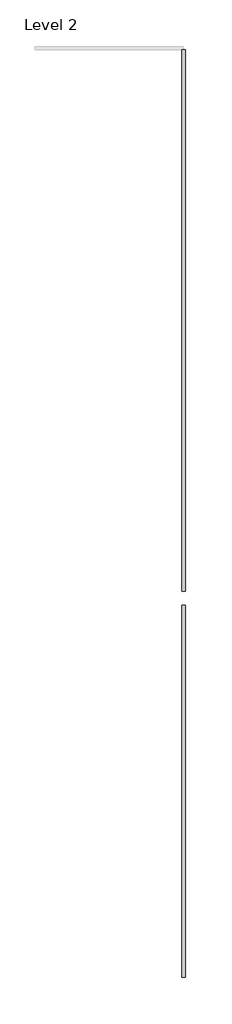
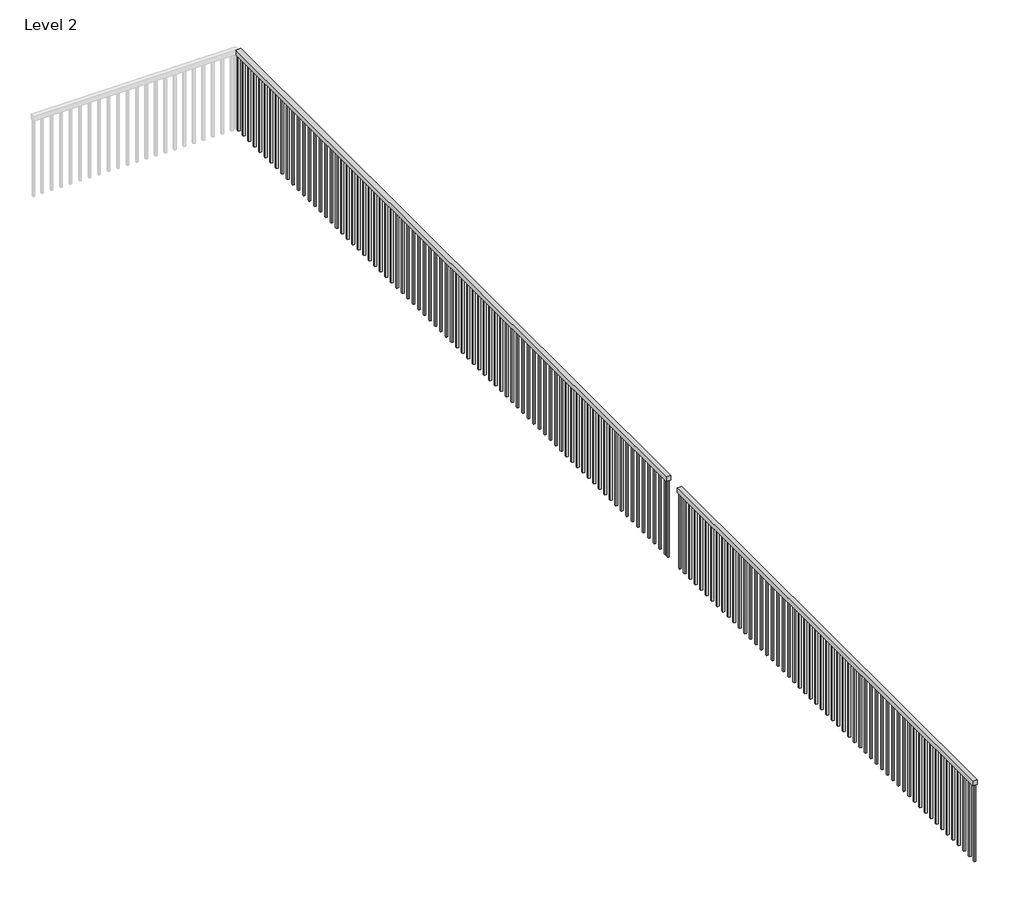
# One storey, part 4 of 5: 2 railings.
"""IFC4 building model written with IfcOpenShell, lengths in millimetres."""

from ifc_helpers import new_model, si_unit, frame, origin, place, context, project, spatial, polyline, outline, extrude, element, save

model = new_model("IFC4")

# Units and contexts
model_context = context("Model", 3, world=origin())
ifc_project = project(units=[si_unit("LENGTHUNIT", "METRE", prefix="MILLI")], contexts=[model_context])

# Site, building, storey
site = spatial("IfcSite", under=ifc_project)
building = spatial("IfcBuilding", under=site)
storey = spatial("IfcBuildingStorey", under=building, Name="Level 2", Elevation=3048.0)

# Railings
placement = place(None, origin())
element("IfcRailing", 1, ObjectType="Handrail - Rectangular", at=placement, inside=storey, context=model_context, shape_type="SweptSolid", body=[
    extrude(outline(polyline([(16296.0289933, 16349.0250499), (16346.8289933, 16349.0250499), (16346.8289933, 8367.8237525), (16296.0289933, 8367.8237525), (16296.0289933, 16349.0250499)])), frame((0.0, 0.0, 3911.6), z_axis=(0.0, 0.0, 1.0), x_axis=(1.0, 0.0, 0.0)), (0.0, 0.0, 1.0), 50.8),
    extrude(outline(polyline([(16311.9039933, 8433.7500499), (16330.9539933, 8433.7500499), (16330.9539933, 8414.7000499), (16311.9039933, 8414.7000499), (16311.9039933, 8433.7500499)])), frame((0.0, 0.0, 3048.0), z_axis=(0.0, 0.0, 1.0), x_axis=(1.0, 0.0, 0.0)), (0.0, 0.0, 1.0), 863.6),
    extrude(outline(polyline([(16311.9039933, 8535.3500499), (16330.9539933, 8535.3500499), (16330.9539933, 8516.3000499), (16311.9039933, 8516.3000499), (16311.9039933, 8535.3500499)])), frame((0.0, 0.0, 3048.0), z_axis=(0.0, 0.0, 1.0), x_axis=(1.0, 0.0, 0.0)), (0.0, 0.0, 1.0), 863.6),
    extrude(outline(polyline([(16311.9039933, 8636.9500499), (16330.9539933, 8636.9500499), (16330.9539933, 8617.9000499), (16311.9039933, 8617.9000499), (16311.9039933, 8636.9500499)])), frame((0.0, 0.0, 3048.0), z_axis=(0.0, 0.0, 1.0), x_axis=(1.0, 0.0, 0.0)), (0.0, 0.0, 1.0), 863.6),
    extrude(outline(polyline([(16311.9039933, 8738.5500499), (16330.9539933, 8738.5500499), (16330.9539933, 8719.5000499), (16311.9039933, 8719.5000499), (16311.9039933, 8738.5500499)])), frame((0.0, 0.0, 3048.0), z_axis=(0.0, 0.0, 1.0), x_axis=(1.0, 0.0, 0.0)), (0.0, 0.0, 1.0), 863.6),
    extrude(outline(polyline([(16311.9039933, 8840.1500499), (16330.9539933, 8840.1500499), (16330.9539933, 8821.1000499), (16311.9039933, 8821.1000499), (16311.9039933, 8840.1500499)])), frame((0.0, 0.0, 3048.0), z_axis=(0.0, 0.0, 1.0), x_axis=(1.0, 0.0, 0.0)), (0.0, 0.0, 1.0), 863.6),
    extrude(outline(polyline([(16311.9039933, 8941.7500499), (16330.9539933, 8941.7500499), (16330.9539933, 8922.7000499), (16311.9039933, 8922.7000499), (16311.9039933, 8941.7500499)])), frame((0.0, 0.0, 3048.0), z_axis=(0.0, 0.0, 1.0), x_axis=(1.0, 0.0, 0.0)), (0.0, 0.0, 1.0), 863.6),
    extrude(outline(polyline([(16311.9039933, 9043.3500499), (16330.9539933, 9043.3500499), (16330.9539933, 9024.3000499), (16311.9039933, 9024.3000499), (16311.9039933, 9043.3500499)])), frame((0.0, 0.0, 3048.0), z_axis=(0.0, 0.0, 1.0), x_axis=(1.0, 0.0, 0.0)), (0.0, 0.0, 1.0), 863.6),
    extrude(outline(polyline([(16311.9039933, 9144.9500499), (16330.9539933, 9144.9500499), (16330.9539933, 9125.9000499), (16311.9039933, 9125.9000499), (16311.9039933, 9144.9500499)])), frame((0.0, 0.0, 3048.0), z_axis=(0.0, 0.0, 1.0), x_axis=(1.0, 0.0, 0.0)), (0.0, 0.0, 1.0), 863.6),
    extrude(outline(polyline([(16311.9039933, 9246.5500499), (16330.9539933, 9246.5500499), (16330.9539933, 9227.5000499), (16311.9039933, 9227.5000499), (16311.9039933, 9246.5500499)])), frame((0.0, 0.0, 3048.0), z_axis=(0.0, 0.0, 1.0), x_axis=(1.0, 0.0, 0.0)), (0.0, 0.0, 1.0), 863.6),
    extrude(outline(polyline([(16311.9039933, 9348.1500499), (16330.9539933, 9348.1500499), (16330.9539933, 9329.1000499), (16311.9039933, 9329.1000499), (16311.9039933, 9348.1500499)])), frame((0.0, 0.0, 3048.0), z_axis=(0.0, 0.0, 1.0), x_axis=(1.0, 0.0, 0.0)), (0.0, 0.0, 1.0), 863.6),
    extrude(outline(polyline([(16311.9039933, 9449.7500499), (16330.9539933, 9449.7500499), (16330.9539933, 9430.7000499), (16311.9039933, 9430.7000499), (16311.9039933, 9449.7500499)])), frame((0.0, 0.0, 3048.0), z_axis=(0.0, 0.0, 1.0), x_axis=(1.0, 0.0, 0.0)), (0.0, 0.0, 1.0), 863.6),
    extrude(outline(polyline([(16311.9039933, 9551.3500499), (16330.9539933, 9551.3500499), (16330.9539933, 9532.3000499), (16311.9039933, 9532.3000499), (16311.9039933, 9551.3500499)])), frame((0.0, 0.0, 3048.0), z_axis=(0.0, 0.0, 1.0), x_axis=(1.0, 0.0, 0.0)), (0.0, 0.0, 1.0), 863.6),
    extrude(outline(polyline([(16311.9039933, 9652.9500499), (16330.9539933, 9652.9500499), (16330.9539933, 9633.9000499), (16311.9039933, 9633.9000499), (16311.9039933, 9652.9500499)])), frame((0.0, 0.0, 3048.0), z_axis=(0.0, 0.0, 1.0), x_axis=(1.0, 0.0, 0.0)), (0.0, 0.0, 1.0), 863.6),
    extrude(outline(polyline([(16311.9039933, 9754.5500499), (16330.9539933, 9754.5500499), (16330.9539933, 9735.5000499), (16311.9039933, 9735.5000499), (16311.9039933, 9754.5500499)])), frame((0.0, 0.0, 3048.0), z_axis=(0.0, 0.0, 1.0), x_axis=(1.0, 0.0, 0.0)), (0.0, 0.0, 1.0), 863.6),
    extrude(outline(polyline([(16311.9039933, 9856.1500499), (16330.9539933, 9856.1500499), (16330.9539933, 9837.1000499), (16311.9039933, 9837.1000499), (16311.9039933, 9856.1500499)])), frame((0.0, 0.0, 3048.0), z_axis=(0.0, 0.0, 1.0), x_axis=(1.0, 0.0, 0.0)), (0.0, 0.0, 1.0), 863.6),
    extrude(outline(polyline([(16311.9039933, 9957.7500499), (16330.9539933, 9957.7500499), (16330.9539933, 9938.7000499), (16311.9039933, 9938.7000499), (16311.9039933, 9957.7500499)])), frame((0.0, 0.0, 3048.0), z_axis=(0.0, 0.0, 1.0), x_axis=(1.0, 0.0, 0.0)), (0.0, 0.0, 1.0), 863.6),
    extrude(outline(polyline([(16311.9039933, 10059.3500499), (16330.9539933, 10059.3500499), (16330.9539933, 10040.3000499), (16311.9039933, 10040.3000499), (16311.9039933, 10059.3500499)])), frame((0.0, 0.0, 3048.0), z_axis=(0.0, 0.0, 1.0), x_axis=(1.0, 0.0, 0.0)), (0.0, 0.0, 1.0), 863.6),
    extrude(outline(polyline([(16311.9039933, 10160.9500499), (16330.9539933, 10160.9500499), (16330.9539933, 10141.9000499), (16311.9039933, 10141.9000499), (16311.9039933, 10160.9500499)])), frame((0.0, 0.0, 3048.0), z_axis=(0.0, 0.0, 1.0), x_axis=(1.0, 0.0, 0.0)), (0.0, 0.0, 1.0), 863.6),
    extrude(outline(polyline([(16311.9039933, 10262.5500499), (16330.9539933, 10262.5500499), (16330.9539933, 10243.5000499), (16311.9039933, 10243.5000499), (16311.9039933, 10262.5500499)])), frame((0.0, 0.0, 3048.0), z_axis=(0.0, 0.0, 1.0), x_axis=(1.0, 0.0, 0.0)), (0.0, 0.0, 1.0), 863.6),
    extrude(outline(polyline([(16311.9039933, 10364.1500499), (16330.9539933, 10364.1500499), (16330.9539933, 10345.1000499), (16311.9039933, 10345.1000499), (16311.9039933, 10364.1500499)])), frame((0.0, 0.0, 3048.0), z_axis=(0.0, 0.0, 1.0), x_axis=(1.0, 0.0, 0.0)), (0.0, 0.0, 1.0), 863.6),
    extrude(outline(polyline([(16311.9039933, 10465.7500499), (16330.9539933, 10465.7500499), (16330.9539933, 10446.7000499), (16311.9039933, 10446.7000499), (16311.9039933, 10465.7500499)])), frame((0.0, 0.0, 3048.0), z_axis=(0.0, 0.0, 1.0), x_axis=(1.0, 0.0, 0.0)), (0.0, 0.0, 1.0), 863.6),
    extrude(outline(polyline([(16311.9039933, 10567.3500499), (16330.9539933, 10567.3500499), (16330.9539933, 10548.3000499), (16311.9039933, 10548.3000499), (16311.9039933, 10567.3500499)])), frame((0.0, 0.0, 3048.0), z_axis=(0.0, 0.0, 1.0), x_axis=(1.0, 0.0, 0.0)), (0.0, 0.0, 1.0), 863.6),
    extrude(outline(polyline([(16311.9039933, 10668.9500499), (16330.9539933, 10668.9500499), (16330.9539933, 10649.9000499), (16311.9039933, 10649.9000499), (16311.9039933, 10668.9500499)])), frame((0.0, 0.0, 3048.0), z_axis=(0.0, 0.0, 1.0), x_axis=(1.0, 0.0, 0.0)), (0.0, 0.0, 1.0), 863.6),
    extrude(outline(polyline([(16311.9039933, 10770.5500499), (16330.9539933, 10770.5500499), (16330.9539933, 10751.5000499), (16311.9039933, 10751.5000499), (16311.9039933, 10770.5500499)])), frame((0.0, 0.0, 3048.0), z_axis=(0.0, 0.0, 1.0), x_axis=(1.0, 0.0, 0.0)), (0.0, 0.0, 1.0), 863.6),
    extrude(outline(polyline([(16311.9039933, 10872.1500499), (16330.9539933, 10872.1500499), (16330.9539933, 10853.1000499), (16311.9039933, 10853.1000499), (16311.9039933, 10872.1500499)])), frame((0.0, 0.0, 3048.0), z_axis=(0.0, 0.0, 1.0), x_axis=(1.0, 0.0, 0.0)), (0.0, 0.0, 1.0), 863.6),
    extrude(outline(polyline([(16311.9039933, 10973.7500499), (16330.9539933, 10973.7500499), (16330.9539933, 10954.7000499), (16311.9039933, 10954.7000499), (16311.9039933, 10973.7500499)])), frame((0.0, 0.0, 3048.0), z_axis=(0.0, 0.0, 1.0), x_axis=(1.0, 0.0, 0.0)), (0.0, 0.0, 1.0), 863.6),
    extrude(outline(polyline([(16311.9039933, 11075.3500499), (16330.9539933, 11075.3500499), (16330.9539933, 11056.3000499), (16311.9039933, 11056.3000499), (16311.9039933, 11075.3500499)])), frame((0.0, 0.0, 3048.0), z_axis=(0.0, 0.0, 1.0), x_axis=(1.0, 0.0, 0.0)), (0.0, 0.0, 1.0), 863.6),
    extrude(outline(polyline([(16311.9039933, 11176.9500499), (16330.9539933, 11176.9500499), (16330.9539933, 11157.9000499), (16311.9039933, 11157.9000499), (16311.9039933, 11176.9500499)])), frame((0.0, 0.0, 3048.0), z_axis=(0.0, 0.0, 1.0), x_axis=(1.0, 0.0, 0.0)), (0.0, 0.0, 1.0), 863.6),
    extrude(outline(polyline([(16311.9039933, 11278.5500499), (16330.9539933, 11278.5500499), (16330.9539933, 11259.5000499), (16311.9039933, 11259.5000499), (16311.9039933, 11278.5500499)])), frame((0.0, 0.0, 3048.0), z_axis=(0.0, 0.0, 1.0), x_axis=(1.0, 0.0, 0.0)), (0.0, 0.0, 1.0), 863.6),
    extrude(outline(polyline([(16311.9039933, 11380.1500499), (16330.9539933, 11380.1500499), (16330.9539933, 11361.1000499), (16311.9039933, 11361.1000499), (16311.9039933, 11380.1500499)])), frame((0.0, 0.0, 3048.0), z_axis=(0.0, 0.0, 1.0), x_axis=(1.0, 0.0, 0.0)), (0.0, 0.0, 1.0), 863.6),
    extrude(outline(polyline([(16311.9039933, 11481.7500499), (16330.9539933, 11481.7500499), (16330.9539933, 11462.7000499), (16311.9039933, 11462.7000499), (16311.9039933, 11481.7500499)])), frame((0.0, 0.0, 3048.0), z_axis=(0.0, 0.0, 1.0), x_axis=(1.0, 0.0, 0.0)), (0.0, 0.0, 1.0), 863.6),
    extrude(outline(polyline([(16311.9039933, 11583.3500499), (16330.9539933, 11583.3500499), (16330.9539933, 11564.3000499), (16311.9039933, 11564.3000499), (16311.9039933, 11583.3500499)])), frame((0.0, 0.0, 3048.0), z_axis=(0.0, 0.0, 1.0), x_axis=(1.0, 0.0, 0.0)), (0.0, 0.0, 1.0), 863.6),
    extrude(outline(polyline([(16311.9039933, 11684.9500499), (16330.9539933, 11684.9500499), (16330.9539933, 11665.9000499), (16311.9039933, 11665.9000499), (16311.9039933, 11684.9500499)])), frame((0.0, 0.0, 3048.0), z_axis=(0.0, 0.0, 1.0), x_axis=(1.0, 0.0, 0.0)), (0.0, 0.0, 1.0), 863.6),
    extrude(outline(polyline([(16311.9039933, 11786.5500499), (16330.9539933, 11786.5500499), (16330.9539933, 11767.5000499), (16311.9039933, 11767.5000499), (16311.9039933, 11786.5500499)])), frame((0.0, 0.0, 3048.0), z_axis=(0.0, 0.0, 1.0), x_axis=(1.0, 0.0, 0.0)), (0.0, 0.0, 1.0), 863.6),
    extrude(outline(polyline([(16311.9039933, 11888.1500499), (16330.9539933, 11888.1500499), (16330.9539933, 11869.1000499), (16311.9039933, 11869.1000499), (16311.9039933, 11888.1500499)])), frame((0.0, 0.0, 3048.0), z_axis=(0.0, 0.0, 1.0), x_axis=(1.0, 0.0, 0.0)), (0.0, 0.0, 1.0), 863.6),
    extrude(outline(polyline([(16311.9039933, 11989.7500499), (16330.9539933, 11989.7500499), (16330.9539933, 11970.7000499), (16311.9039933, 11970.7000499), (16311.9039933, 11989.7500499)])), frame((0.0, 0.0, 3048.0), z_axis=(0.0, 0.0, 1.0), x_axis=(1.0, 0.0, 0.0)), (0.0, 0.0, 1.0), 863.6),
    extrude(outline(polyline([(16311.9039933, 12091.3500499), (16330.9539933, 12091.3500499), (16330.9539933, 12072.3000499), (16311.9039933, 12072.3000499), (16311.9039933, 12091.3500499)])), frame((0.0, 0.0, 3048.0), z_axis=(0.0, 0.0, 1.0), x_axis=(1.0, 0.0, 0.0)), (0.0, 0.0, 1.0), 863.6),
    extrude(outline(polyline([(16311.9039933, 12192.9500499), (16330.9539933, 12192.9500499), (16330.9539933, 12173.9000499), (16311.9039933, 12173.9000499), (16311.9039933, 12192.9500499)])), frame((0.0, 0.0, 3048.0), z_axis=(0.0, 0.0, 1.0), x_axis=(1.0, 0.0, 0.0)), (0.0, 0.0, 1.0), 863.6),
    extrude(outline(polyline([(16311.9039933, 12294.5500499), (16330.9539933, 12294.5500499), (16330.9539933, 12275.5000499), (16311.9039933, 12275.5000499), (16311.9039933, 12294.5500499)])), frame((0.0, 0.0, 3048.0), z_axis=(0.0, 0.0, 1.0), x_axis=(1.0, 0.0, 0.0)), (0.0, 0.0, 1.0), 863.6),
    extrude(outline(polyline([(16311.9039933, 12396.1500499), (16330.9539933, 12396.1500499), (16330.9539933, 12377.1000499), (16311.9039933, 12377.1000499), (16311.9039933, 12396.1500499)])), frame((0.0, 0.0, 3048.0), z_axis=(0.0, 0.0, 1.0), x_axis=(1.0, 0.0, 0.0)), (0.0, 0.0, 1.0), 863.6),
    extrude(outline(polyline([(16311.9039933, 12497.7500499), (16330.9539933, 12497.7500499), (16330.9539933, 12478.7000499), (16311.9039933, 12478.7000499), (16311.9039933, 12497.7500499)])), frame((0.0, 0.0, 3048.0), z_axis=(0.0, 0.0, 1.0), x_axis=(1.0, 0.0, 0.0)), (0.0, 0.0, 1.0), 863.6),
    extrude(outline(polyline([(16311.9039933, 12599.3500499), (16330.9539933, 12599.3500499), (16330.9539933, 12580.3000499), (16311.9039933, 12580.3000499), (16311.9039933, 12599.3500499)])), frame((0.0, 0.0, 3048.0), z_axis=(0.0, 0.0, 1.0), x_axis=(1.0, 0.0, 0.0)), (0.0, 0.0, 1.0), 863.6),
    extrude(outline(polyline([(16311.9039933, 12700.9500499), (16330.9539933, 12700.9500499), (16330.9539933, 12681.9000499), (16311.9039933, 12681.9000499), (16311.9039933, 12700.9500499)])), frame((0.0, 0.0, 3048.0), z_axis=(0.0, 0.0, 1.0), x_axis=(1.0, 0.0, 0.0)), (0.0, 0.0, 1.0), 863.6),
    extrude(outline(polyline([(16311.9039933, 12802.5500499), (16330.9539933, 12802.5500499), (16330.9539933, 12783.5000499), (16311.9039933, 12783.5000499), (16311.9039933, 12802.5500499)])), frame((0.0, 0.0, 3048.0), z_axis=(0.0, 0.0, 1.0), x_axis=(1.0, 0.0, 0.0)), (0.0, 0.0, 1.0), 863.6),
    extrude(outline(polyline([(16311.9039933, 12904.1500499), (16330.9539933, 12904.1500499), (16330.9539933, 12885.1000499), (16311.9039933, 12885.1000499), (16311.9039933, 12904.1500499)])), frame((0.0, 0.0, 3048.0), z_axis=(0.0, 0.0, 1.0), x_axis=(1.0, 0.0, 0.0)), (0.0, 0.0, 1.0), 863.6),
    extrude(outline(polyline([(16311.9039933, 13005.7500499), (16330.9539933, 13005.7500499), (16330.9539933, 12986.7000499), (16311.9039933, 12986.7000499), (16311.9039933, 13005.7500499)])), frame((0.0, 0.0, 3048.0), z_axis=(0.0, 0.0, 1.0), x_axis=(1.0, 0.0, 0.0)), (0.0, 0.0, 1.0), 863.6),
    extrude(outline(polyline([(16311.9039933, 13107.3500499), (16330.9539933, 13107.3500499), (16330.9539933, 13088.3000499), (16311.9039933, 13088.3000499), (16311.9039933, 13107.3500499)])), frame((0.0, 0.0, 3048.0), z_axis=(0.0, 0.0, 1.0), x_axis=(1.0, 0.0, 0.0)), (0.0, 0.0, 1.0), 863.6),
    extrude(outline(polyline([(16311.9039933, 13208.9500499), (16330.9539933, 13208.9500499), (16330.9539933, 13189.9000499), (16311.9039933, 13189.9000499), (16311.9039933, 13208.9500499)])), frame((0.0, 0.0, 3048.0), z_axis=(0.0, 0.0, 1.0), x_axis=(1.0, 0.0, 0.0)), (0.0, 0.0, 1.0), 863.6),
    extrude(outline(polyline([(16311.9039933, 13310.5500499), (16330.9539933, 13310.5500499), (16330.9539933, 13291.5000499), (16311.9039933, 13291.5000499), (16311.9039933, 13310.5500499)])), frame((0.0, 0.0, 3048.0), z_axis=(0.0, 0.0, 1.0), x_axis=(1.0, 0.0, 0.0)), (0.0, 0.0, 1.0), 863.6),
    extrude(outline(polyline([(16311.9039933, 13412.1500499), (16330.9539933, 13412.1500499), (16330.9539933, 13393.1000499), (16311.9039933, 13393.1000499), (16311.9039933, 13412.1500499)])), frame((0.0, 0.0, 3048.0), z_axis=(0.0, 0.0, 1.0), x_axis=(1.0, 0.0, 0.0)), (0.0, 0.0, 1.0), 863.6),
    extrude(outline(polyline([(16311.9039933, 13513.7500499), (16330.9539933, 13513.7500499), (16330.9539933, 13494.7000499), (16311.9039933, 13494.7000499), (16311.9039933, 13513.7500499)])), frame((0.0, 0.0, 3048.0), z_axis=(0.0, 0.0, 1.0), x_axis=(1.0, 0.0, 0.0)), (0.0, 0.0, 1.0), 863.6),
    extrude(outline(polyline([(16311.9039933, 13615.3500499), (16330.9539933, 13615.3500499), (16330.9539933, 13596.3000499), (16311.9039933, 13596.3000499), (16311.9039933, 13615.3500499)])), frame((0.0, 0.0, 3048.0), z_axis=(0.0, 0.0, 1.0), x_axis=(1.0, 0.0, 0.0)), (0.0, 0.0, 1.0), 863.6),
    extrude(outline(polyline([(16311.9039933, 13716.9500499), (16330.9539933, 13716.9500499), (16330.9539933, 13697.9000499), (16311.9039933, 13697.9000499), (16311.9039933, 13716.9500499)])), frame((0.0, 0.0, 3048.0), z_axis=(0.0, 0.0, 1.0), x_axis=(1.0, 0.0, 0.0)), (0.0, 0.0, 1.0), 863.6),
    extrude(outline(polyline([(16311.9039933, 13818.5500499), (16330.9539933, 13818.5500499), (16330.9539933, 13799.5000499), (16311.9039933, 13799.5000499), (16311.9039933, 13818.5500499)])), frame((0.0, 0.0, 3048.0), z_axis=(0.0, 0.0, 1.0), x_axis=(1.0, 0.0, 0.0)), (0.0, 0.0, 1.0), 863.6),
    extrude(outline(polyline([(16311.9039933, 13920.1500499), (16330.9539933, 13920.1500499), (16330.9539933, 13901.1000499), (16311.9039933, 13901.1000499), (16311.9039933, 13920.1500499)])), frame((0.0, 0.0, 3048.0), z_axis=(0.0, 0.0, 1.0), x_axis=(1.0, 0.0, 0.0)), (0.0, 0.0, 1.0), 863.6),
    extrude(outline(polyline([(16311.9039933, 14021.7500499), (16330.9539933, 14021.7500499), (16330.9539933, 14002.7000499), (16311.9039933, 14002.7000499), (16311.9039933, 14021.7500499)])), frame((0.0, 0.0, 3048.0), z_axis=(0.0, 0.0, 1.0), x_axis=(1.0, 0.0, 0.0)), (0.0, 0.0, 1.0), 863.6),
    extrude(outline(polyline([(16311.9039933, 14123.3500499), (16330.9539933, 14123.3500499), (16330.9539933, 14104.3000499), (16311.9039933, 14104.3000499), (16311.9039933, 14123.3500499)])), frame((0.0, 0.0, 3048.0), z_axis=(0.0, 0.0, 1.0), x_axis=(1.0, 0.0, 0.0)), (0.0, 0.0, 1.0), 863.6),
    extrude(outline(polyline([(16311.9039933, 14224.9500499), (16330.9539933, 14224.9500499), (16330.9539933, 14205.9000499), (16311.9039933, 14205.9000499), (16311.9039933, 14224.9500499)])), frame((0.0, 0.0, 3048.0), z_axis=(0.0, 0.0, 1.0), x_axis=(1.0, 0.0, 0.0)), (0.0, 0.0, 1.0), 863.6),
    extrude(outline(polyline([(16311.9039933, 14326.5500499), (16330.9539933, 14326.5500499), (16330.9539933, 14307.5000499), (16311.9039933, 14307.5000499), (16311.9039933, 14326.5500499)])), frame((0.0, 0.0, 3048.0), z_axis=(0.0, 0.0, 1.0), x_axis=(1.0, 0.0, 0.0)), (0.0, 0.0, 1.0), 863.6),
    extrude(outline(polyline([(16311.9039933, 14428.1500499), (16330.9539933, 14428.1500499), (16330.9539933, 14409.1000499), (16311.9039933, 14409.1000499), (16311.9039933, 14428.1500499)])), frame((0.0, 0.0, 3048.0), z_axis=(0.0, 0.0, 1.0), x_axis=(1.0, 0.0, 0.0)), (0.0, 0.0, 1.0), 863.6),
    extrude(outline(polyline([(16311.9039933, 14529.7500499), (16330.9539933, 14529.7500499), (16330.9539933, 14510.7000499), (16311.9039933, 14510.7000499), (16311.9039933, 14529.7500499)])), frame((0.0, 0.0, 3048.0), z_axis=(0.0, 0.0, 1.0), x_axis=(1.0, 0.0, 0.0)), (0.0, 0.0, 1.0), 863.6),
    extrude(outline(polyline([(16311.9039933, 14631.3500499), (16330.9539933, 14631.3500499), (16330.9539933, 14612.3000499), (16311.9039933, 14612.3000499), (16311.9039933, 14631.3500499)])), frame((0.0, 0.0, 3048.0), z_axis=(0.0, 0.0, 1.0), x_axis=(1.0, 0.0, 0.0)), (0.0, 0.0, 1.0), 863.6),
    extrude(outline(polyline([(16311.9039933, 14732.9500499), (16330.9539933, 14732.9500499), (16330.9539933, 14713.9000499), (16311.9039933, 14713.9000499), (16311.9039933, 14732.9500499)])), frame((0.0, 0.0, 3048.0), z_axis=(0.0, 0.0, 1.0), x_axis=(1.0, 0.0, 0.0)), (0.0, 0.0, 1.0), 863.6),
    extrude(outline(polyline([(16311.9039933, 14834.5500499), (16330.9539933, 14834.5500499), (16330.9539933, 14815.5000499), (16311.9039933, 14815.5000499), (16311.9039933, 14834.5500499)])), frame((0.0, 0.0, 3048.0), z_axis=(0.0, 0.0, 1.0), x_axis=(1.0, 0.0, 0.0)), (0.0, 0.0, 1.0), 863.6),
    extrude(outline(polyline([(16311.9039933, 14936.1500499), (16330.9539933, 14936.1500499), (16330.9539933, 14917.1000499), (16311.9039933, 14917.1000499), (16311.9039933, 14936.1500499)])), frame((0.0, 0.0, 3048.0), z_axis=(0.0, 0.0, 1.0), x_axis=(1.0, 0.0, 0.0)), (0.0, 0.0, 1.0), 863.6),
    extrude(outline(polyline([(16311.9039933, 15037.7500499), (16330.9539933, 15037.7500499), (16330.9539933, 15018.7000499), (16311.9039933, 15018.7000499), (16311.9039933, 15037.7500499)])), frame((0.0, 0.0, 3048.0), z_axis=(0.0, 0.0, 1.0), x_axis=(1.0, 0.0, 0.0)), (0.0, 0.0, 1.0), 863.6),
    extrude(outline(polyline([(16311.9039933, 15139.3500499), (16330.9539933, 15139.3500499), (16330.9539933, 15120.3000499), (16311.9039933, 15120.3000499), (16311.9039933, 15139.3500499)])), frame((0.0, 0.0, 3048.0), z_axis=(0.0, 0.0, 1.0), x_axis=(1.0, 0.0, 0.0)), (0.0, 0.0, 1.0), 863.6),
    extrude(outline(polyline([(16311.9039933, 15240.9500499), (16330.9539933, 15240.9500499), (16330.9539933, 15221.9000499), (16311.9039933, 15221.9000499), (16311.9039933, 15240.9500499)])), frame((0.0, 0.0, 3048.0), z_axis=(0.0, 0.0, 1.0), x_axis=(1.0, 0.0, 0.0)), (0.0, 0.0, 1.0), 863.6),
    extrude(outline(polyline([(16311.9039933, 15342.5500499), (16330.9539933, 15342.5500499), (16330.9539933, 15323.5000499), (16311.9039933, 15323.5000499), (16311.9039933, 15342.5500499)])), frame((0.0, 0.0, 3048.0), z_axis=(0.0, 0.0, 1.0), x_axis=(1.0, 0.0, 0.0)), (0.0, 0.0, 1.0), 863.6),
    extrude(outline(polyline([(16311.9039933, 15444.1500499), (16330.9539933, 15444.1500499), (16330.9539933, 15425.1000499), (16311.9039933, 15425.1000499), (16311.9039933, 15444.1500499)])), frame((0.0, 0.0, 3048.0), z_axis=(0.0, 0.0, 1.0), x_axis=(1.0, 0.0, 0.0)), (0.0, 0.0, 1.0), 863.6),
    extrude(outline(polyline([(16311.9039933, 15545.7500499), (16330.9539933, 15545.7500499), (16330.9539933, 15526.7000499), (16311.9039933, 15526.7000499), (16311.9039933, 15545.7500499)])), frame((0.0, 0.0, 3048.0), z_axis=(0.0, 0.0, 1.0), x_axis=(1.0, 0.0, 0.0)), (0.0, 0.0, 1.0), 863.6),
    extrude(outline(polyline([(16311.9039933, 15647.3500499), (16330.9539933, 15647.3500499), (16330.9539933, 15628.3000499), (16311.9039933, 15628.3000499), (16311.9039933, 15647.3500499)])), frame((0.0, 0.0, 3048.0), z_axis=(0.0, 0.0, 1.0), x_axis=(1.0, 0.0, 0.0)), (0.0, 0.0, 1.0), 863.6),
    extrude(outline(polyline([(16311.9039933, 15748.9500499), (16330.9539933, 15748.9500499), (16330.9539933, 15729.9000499), (16311.9039933, 15729.9000499), (16311.9039933, 15748.9500499)])), frame((0.0, 0.0, 3048.0), z_axis=(0.0, 0.0, 1.0), x_axis=(1.0, 0.0, 0.0)), (0.0, 0.0, 1.0), 863.6),
    extrude(outline(polyline([(16311.9039933, 15850.5500499), (16330.9539933, 15850.5500499), (16330.9539933, 15831.5000499), (16311.9039933, 15831.5000499), (16311.9039933, 15850.5500499)])), frame((0.0, 0.0, 3048.0), z_axis=(0.0, 0.0, 1.0), x_axis=(1.0, 0.0, 0.0)), (0.0, 0.0, 1.0), 863.6),
    extrude(outline(polyline([(16311.9039933, 15952.1500499), (16330.9539933, 15952.1500499), (16330.9539933, 15933.1000499), (16311.9039933, 15933.1000499), (16311.9039933, 15952.1500499)])), frame((0.0, 0.0, 3048.0), z_axis=(0.0, 0.0, 1.0), x_axis=(1.0, 0.0, 0.0)), (0.0, 0.0, 1.0), 863.6),
    extrude(outline(polyline([(16311.9039933, 16053.7500499), (16330.9539933, 16053.7500499), (16330.9539933, 16034.7000499), (16311.9039933, 16034.7000499), (16311.9039933, 16053.7500499)])), frame((0.0, 0.0, 3048.0), z_axis=(0.0, 0.0, 1.0), x_axis=(1.0, 0.0, 0.0)), (0.0, 0.0, 1.0), 863.6),
    extrude(outline(polyline([(16311.9039933, 16155.3500499), (16330.9539933, 16155.3500499), (16330.9539933, 16136.3000499), (16311.9039933, 16136.3000499), (16311.9039933, 16155.3500499)])), frame((0.0, 0.0, 3048.0), z_axis=(0.0, 0.0, 1.0), x_axis=(1.0, 0.0, 0.0)), (0.0, 0.0, 1.0), 863.6),
    extrude(outline(polyline([(16311.9039933, 16256.9500499), (16330.9539933, 16256.9500499), (16330.9539933, 16237.9000499), (16311.9039933, 16237.9000499), (16311.9039933, 16256.9500499)])), frame((0.0, 0.0, 3048.0), z_axis=(0.0, 0.0, 1.0), x_axis=(1.0, 0.0, 0.0)), (0.0, 0.0, 1.0), 863.6),
    extrude(outline(polyline([(16311.9039933, 8386.8737525), (16330.9539933, 8386.8737525), (16330.9539933, 8367.8237525), (16311.9039933, 8367.8237525), (16311.9039933, 8386.8737525)])), frame((0.0, 0.0, 3048.0), z_axis=(0.0, 0.0, 1.0), x_axis=(1.0, 0.0, 0.0)), (0.0, 0.0, 1.0), 863.6),
    extrude(outline(polyline([(16311.9039933, 16349.0250499), (16330.9539933, 16349.0250499), (16330.9539933, 16329.9750499), (16311.9039933, 16329.9750499), (16311.9039933, 16349.0250499)])), frame((0.0, 0.0, 3048.0), z_axis=(0.0, 0.0, 1.0), x_axis=(1.0, 0.0, 0.0)), (0.0, 0.0, 1.0), 863.6),
])
element("IfcRailing", 2, ObjectType="Handrail - Rectangular", at=placement, inside=storey, context=model_context, shape_type="SweptSolid", body=[
    extrude(outline(polyline([(16296.0289933, 8164.6237525), (16346.8289933, 8164.6237525), (16346.8289933, 2678.2237525), (16296.0289933, 2678.2237525), (16296.0289933, 8164.6237525)])), frame((0.0, 0.0, 3911.6), z_axis=(0.0, 0.0, 1.0), x_axis=(1.0, 0.0, 0.0)), (0.0, 0.0, 1.0), 50.8),
    extrude(outline(polyline([(16311.9039933, 2789.3487525), (16330.9539933, 2789.3487525), (16330.9539933, 2770.2987525), (16311.9039933, 2770.2987525), (16311.9039933, 2789.3487525)])), frame((0.0, 0.0, 3048.0), z_axis=(0.0, 0.0, 1.0), x_axis=(1.0, 0.0, 0.0)), (0.0, 0.0, 1.0), 863.6),
    extrude(outline(polyline([(16311.9039933, 2890.9487525), (16330.9539933, 2890.9487525), (16330.9539933, 2871.8987525), (16311.9039933, 2871.8987525), (16311.9039933, 2890.9487525)])), frame((0.0, 0.0, 3048.0), z_axis=(0.0, 0.0, 1.0), x_axis=(1.0, 0.0, 0.0)), (0.0, 0.0, 1.0), 863.6),
    extrude(outline(polyline([(16311.9039933, 2992.5487525), (16330.9539933, 2992.5487525), (16330.9539933, 2973.4987525), (16311.9039933, 2973.4987525), (16311.9039933, 2992.5487525)])), frame((0.0, 0.0, 3048.0), z_axis=(0.0, 0.0, 1.0), x_axis=(1.0, 0.0, 0.0)), (0.0, 0.0, 1.0), 863.6),
    extrude(outline(polyline([(16311.9039933, 3094.1487525), (16330.9539933, 3094.1487525), (16330.9539933, 3075.0987525), (16311.9039933, 3075.0987525), (16311.9039933, 3094.1487525)])), frame((0.0, 0.0, 3048.0), z_axis=(0.0, 0.0, 1.0), x_axis=(1.0, 0.0, 0.0)), (0.0, 0.0, 1.0), 863.6),
    extrude(outline(polyline([(16311.9039933, 3195.7487525), (16330.9539933, 3195.7487525), (16330.9539933, 3176.6987525), (16311.9039933, 3176.6987525), (16311.9039933, 3195.7487525)])), frame((0.0, 0.0, 3048.0), z_axis=(0.0, 0.0, 1.0), x_axis=(1.0, 0.0, 0.0)), (0.0, 0.0, 1.0), 863.6),
    extrude(outline(polyline([(16311.9039933, 3297.3487525), (16330.9539933, 3297.3487525), (16330.9539933, 3278.2987525), (16311.9039933, 3278.2987525), (16311.9039933, 3297.3487525)])), frame((0.0, 0.0, 3048.0), z_axis=(0.0, 0.0, 1.0), x_axis=(1.0, 0.0, 0.0)), (0.0, 0.0, 1.0), 863.6),
    extrude(outline(polyline([(16311.9039933, 3398.9487525), (16330.9539933, 3398.9487525), (16330.9539933, 3379.8987525), (16311.9039933, 3379.8987525), (16311.9039933, 3398.9487525)])), frame((0.0, 0.0, 3048.0), z_axis=(0.0, 0.0, 1.0), x_axis=(1.0, 0.0, 0.0)), (0.0, 0.0, 1.0), 863.6),
    extrude(outline(polyline([(16311.9039933, 3500.5487525), (16330.9539933, 3500.5487525), (16330.9539933, 3481.4987525), (16311.9039933, 3481.4987525), (16311.9039933, 3500.5487525)])), frame((0.0, 0.0, 3048.0), z_axis=(0.0, 0.0, 1.0), x_axis=(1.0, 0.0, 0.0)), (0.0, 0.0, 1.0), 863.6),
    extrude(outline(polyline([(16311.9039933, 3602.1487525), (16330.9539933, 3602.1487525), (16330.9539933, 3583.0987525), (16311.9039933, 3583.0987525), (16311.9039933, 3602.1487525)])), frame((0.0, 0.0, 3048.0), z_axis=(0.0, 0.0, 1.0), x_axis=(1.0, 0.0, 0.0)), (0.0, 0.0, 1.0), 863.6),
    extrude(outline(polyline([(16311.9039933, 3703.7487525), (16330.9539933, 3703.7487525), (16330.9539933, 3684.6987525), (16311.9039933, 3684.6987525), (16311.9039933, 3703.7487525)])), frame((0.0, 0.0, 3048.0), z_axis=(0.0, 0.0, 1.0), x_axis=(1.0, 0.0, 0.0)), (0.0, 0.0, 1.0), 863.6),
    extrude(outline(polyline([(16311.9039933, 3805.3487525), (16330.9539933, 3805.3487525), (16330.9539933, 3786.2987525), (16311.9039933, 3786.2987525), (16311.9039933, 3805.3487525)])), frame((0.0, 0.0, 3048.0), z_axis=(0.0, 0.0, 1.0), x_axis=(1.0, 0.0, 0.0)), (0.0, 0.0, 1.0), 863.6),
    extrude(outline(polyline([(16311.9039933, 3906.9487525), (16330.9539933, 3906.9487525), (16330.9539933, 3887.8987525), (16311.9039933, 3887.8987525), (16311.9039933, 3906.9487525)])), frame((0.0, 0.0, 3048.0), z_axis=(0.0, 0.0, 1.0), x_axis=(1.0, 0.0, 0.0)), (0.0, 0.0, 1.0), 863.6),
    extrude(outline(polyline([(16311.9039933, 4008.5487525), (16330.9539933, 4008.5487525), (16330.9539933, 3989.4987525), (16311.9039933, 3989.4987525), (16311.9039933, 4008.5487525)])), frame((0.0, 0.0, 3048.0), z_axis=(0.0, 0.0, 1.0), x_axis=(1.0, 0.0, 0.0)), (0.0, 0.0, 1.0), 863.6),
    extrude(outline(polyline([(16311.9039933, 4110.1487525), (16330.9539933, 4110.1487525), (16330.9539933, 4091.0987525), (16311.9039933, 4091.0987525), (16311.9039933, 4110.1487525)])), frame((0.0, 0.0, 3048.0), z_axis=(0.0, 0.0, 1.0), x_axis=(1.0, 0.0, 0.0)), (0.0, 0.0, 1.0), 863.6),
    extrude(outline(polyline([(16311.9039933, 4211.7487525), (16330.9539933, 4211.7487525), (16330.9539933, 4192.6987525), (16311.9039933, 4192.6987525), (16311.9039933, 4211.7487525)])), frame((0.0, 0.0, 3048.0), z_axis=(0.0, 0.0, 1.0), x_axis=(1.0, 0.0, 0.0)), (0.0, 0.0, 1.0), 863.6),
    extrude(outline(polyline([(16311.9039933, 4313.3487525), (16330.9539933, 4313.3487525), (16330.9539933, 4294.2987525), (16311.9039933, 4294.2987525), (16311.9039933, 4313.3487525)])), frame((0.0, 0.0, 3048.0), z_axis=(0.0, 0.0, 1.0), x_axis=(1.0, 0.0, 0.0)), (0.0, 0.0, 1.0), 863.6),
    extrude(outline(polyline([(16311.9039933, 4414.9487525), (16330.9539933, 4414.9487525), (16330.9539933, 4395.8987525), (16311.9039933, 4395.8987525), (16311.9039933, 4414.9487525)])), frame((0.0, 0.0, 3048.0), z_axis=(0.0, 0.0, 1.0), x_axis=(1.0, 0.0, 0.0)), (0.0, 0.0, 1.0), 863.6),
    extrude(outline(polyline([(16311.9039933, 4516.5487525), (16330.9539933, 4516.5487525), (16330.9539933, 4497.4987525), (16311.9039933, 4497.4987525), (16311.9039933, 4516.5487525)])), frame((0.0, 0.0, 3048.0), z_axis=(0.0, 0.0, 1.0), x_axis=(1.0, 0.0, 0.0)), (0.0, 0.0, 1.0), 863.6),
    extrude(outline(polyline([(16311.9039933, 4618.1487525), (16330.9539933, 4618.1487525), (16330.9539933, 4599.0987525), (16311.9039933, 4599.0987525), (16311.9039933, 4618.1487525)])), frame((0.0, 0.0, 3048.0), z_axis=(0.0, 0.0, 1.0), x_axis=(1.0, 0.0, 0.0)), (0.0, 0.0, 1.0), 863.6),
    extrude(outline(polyline([(16311.9039933, 4719.7487525), (16330.9539933, 4719.7487525), (16330.9539933, 4700.6987525), (16311.9039933, 4700.6987525), (16311.9039933, 4719.7487525)])), frame((0.0, 0.0, 3048.0), z_axis=(0.0, 0.0, 1.0), x_axis=(1.0, 0.0, 0.0)), (0.0, 0.0, 1.0), 863.6),
    extrude(outline(polyline([(16311.9039933, 4821.3487525), (16330.9539933, 4821.3487525), (16330.9539933, 4802.2987525), (16311.9039933, 4802.2987525), (16311.9039933, 4821.3487525)])), frame((0.0, 0.0, 3048.0), z_axis=(0.0, 0.0, 1.0), x_axis=(1.0, 0.0, 0.0)), (0.0, 0.0, 1.0), 863.6),
    extrude(outline(polyline([(16311.9039933, 4922.9487525), (16330.9539933, 4922.9487525), (16330.9539933, 4903.8987525), (16311.9039933, 4903.8987525), (16311.9039933, 4922.9487525)])), frame((0.0, 0.0, 3048.0), z_axis=(0.0, 0.0, 1.0), x_axis=(1.0, 0.0, 0.0)), (0.0, 0.0, 1.0), 863.6),
    extrude(outline(polyline([(16311.9039933, 5024.5487525), (16330.9539933, 5024.5487525), (16330.9539933, 5005.4987525), (16311.9039933, 5005.4987525), (16311.9039933, 5024.5487525)])), frame((0.0, 0.0, 3048.0), z_axis=(0.0, 0.0, 1.0), x_axis=(1.0, 0.0, 0.0)), (0.0, 0.0, 1.0), 863.6),
    extrude(outline(polyline([(16311.9039933, 5126.1487525), (16330.9539933, 5126.1487525), (16330.9539933, 5107.0987525), (16311.9039933, 5107.0987525), (16311.9039933, 5126.1487525)])), frame((0.0, 0.0, 3048.0), z_axis=(0.0, 0.0, 1.0), x_axis=(1.0, 0.0, 0.0)), (0.0, 0.0, 1.0), 863.6),
    extrude(outline(polyline([(16311.9039933, 5227.7487525), (16330.9539933, 5227.7487525), (16330.9539933, 5208.6987525), (16311.9039933, 5208.6987525), (16311.9039933, 5227.7487525)])), frame((0.0, 0.0, 3048.0), z_axis=(0.0, 0.0, 1.0), x_axis=(1.0, 0.0, 0.0)), (0.0, 0.0, 1.0), 863.6),
    extrude(outline(polyline([(16311.9039933, 5329.3487525), (16330.9539933, 5329.3487525), (16330.9539933, 5310.2987525), (16311.9039933, 5310.2987525), (16311.9039933, 5329.3487525)])), frame((0.0, 0.0, 3048.0), z_axis=(0.0, 0.0, 1.0), x_axis=(1.0, 0.0, 0.0)), (0.0, 0.0, 1.0), 863.6),
    extrude(outline(polyline([(16311.9039933, 5430.9487525), (16330.9539933, 5430.9487525), (16330.9539933, 5411.8987525), (16311.9039933, 5411.8987525), (16311.9039933, 5430.9487525)])), frame((0.0, 0.0, 3048.0), z_axis=(0.0, 0.0, 1.0), x_axis=(1.0, 0.0, 0.0)), (0.0, 0.0, 1.0), 863.6),
    extrude(outline(polyline([(16311.9039933, 5532.5487525), (16330.9539933, 5532.5487525), (16330.9539933, 5513.4987525), (16311.9039933, 5513.4987525), (16311.9039933, 5532.5487525)])), frame((0.0, 0.0, 3048.0), z_axis=(0.0, 0.0, 1.0), x_axis=(1.0, 0.0, 0.0)), (0.0, 0.0, 1.0), 863.6),
    extrude(outline(polyline([(16311.9039933, 5634.1487525), (16330.9539933, 5634.1487525), (16330.9539933, 5615.0987525), (16311.9039933, 5615.0987525), (16311.9039933, 5634.1487525)])), frame((0.0, 0.0, 3048.0), z_axis=(0.0, 0.0, 1.0), x_axis=(1.0, 0.0, 0.0)), (0.0, 0.0, 1.0), 863.6),
    extrude(outline(polyline([(16311.9039933, 5735.7487525), (16330.9539933, 5735.7487525), (16330.9539933, 5716.6987525), (16311.9039933, 5716.6987525), (16311.9039933, 5735.7487525)])), frame((0.0, 0.0, 3048.0), z_axis=(0.0, 0.0, 1.0), x_axis=(1.0, 0.0, 0.0)), (0.0, 0.0, 1.0), 863.6),
    extrude(outline(polyline([(16311.9039933, 5837.3487525), (16330.9539933, 5837.3487525), (16330.9539933, 5818.2987525), (16311.9039933, 5818.2987525), (16311.9039933, 5837.3487525)])), frame((0.0, 0.0, 3048.0), z_axis=(0.0, 0.0, 1.0), x_axis=(1.0, 0.0, 0.0)), (0.0, 0.0, 1.0), 863.6),
    extrude(outline(polyline([(16311.9039933, 5938.9487525), (16330.9539933, 5938.9487525), (16330.9539933, 5919.8987525), (16311.9039933, 5919.8987525), (16311.9039933, 5938.9487525)])), frame((0.0, 0.0, 3048.0), z_axis=(0.0, 0.0, 1.0), x_axis=(1.0, 0.0, 0.0)), (0.0, 0.0, 1.0), 863.6),
    extrude(outline(polyline([(16311.9039933, 6040.5487525), (16330.9539933, 6040.5487525), (16330.9539933, 6021.4987525), (16311.9039933, 6021.4987525), (16311.9039933, 6040.5487525)])), frame((0.0, 0.0, 3048.0), z_axis=(0.0, 0.0, 1.0), x_axis=(1.0, 0.0, 0.0)), (0.0, 0.0, 1.0), 863.6),
    extrude(outline(polyline([(16311.9039933, 6142.1487525), (16330.9539933, 6142.1487525), (16330.9539933, 6123.0987525), (16311.9039933, 6123.0987525), (16311.9039933, 6142.1487525)])), frame((0.0, 0.0, 3048.0), z_axis=(0.0, 0.0, 1.0), x_axis=(1.0, 0.0, 0.0)), (0.0, 0.0, 1.0), 863.6),
    extrude(outline(polyline([(16311.9039933, 6243.7487525), (16330.9539933, 6243.7487525), (16330.9539933, 6224.6987525), (16311.9039933, 6224.6987525), (16311.9039933, 6243.7487525)])), frame((0.0, 0.0, 3048.0), z_axis=(0.0, 0.0, 1.0), x_axis=(1.0, 0.0, 0.0)), (0.0, 0.0, 1.0), 863.6),
    extrude(outline(polyline([(16311.9039933, 6345.3487525), (16330.9539933, 6345.3487525), (16330.9539933, 6326.2987525), (16311.9039933, 6326.2987525), (16311.9039933, 6345.3487525)])), frame((0.0, 0.0, 3048.0), z_axis=(0.0, 0.0, 1.0), x_axis=(1.0, 0.0, 0.0)), (0.0, 0.0, 1.0), 863.6),
    extrude(outline(polyline([(16311.9039933, 6446.9487525), (16330.9539933, 6446.9487525), (16330.9539933, 6427.8987525), (16311.9039933, 6427.8987525), (16311.9039933, 6446.9487525)])), frame((0.0, 0.0, 3048.0), z_axis=(0.0, 0.0, 1.0), x_axis=(1.0, 0.0, 0.0)), (0.0, 0.0, 1.0), 863.6),
    extrude(outline(polyline([(16311.9039933, 6548.5487525), (16330.9539933, 6548.5487525), (16330.9539933, 6529.4987525), (16311.9039933, 6529.4987525), (16311.9039933, 6548.5487525)])), frame((0.0, 0.0, 3048.0), z_axis=(0.0, 0.0, 1.0), x_axis=(1.0, 0.0, 0.0)), (0.0, 0.0, 1.0), 863.6),
    extrude(outline(polyline([(16311.9039933, 6650.1487525), (16330.9539933, 6650.1487525), (16330.9539933, 6631.0987525), (16311.9039933, 6631.0987525), (16311.9039933, 6650.1487525)])), frame((0.0, 0.0, 3048.0), z_axis=(0.0, 0.0, 1.0), x_axis=(1.0, 0.0, 0.0)), (0.0, 0.0, 1.0), 863.6),
    extrude(outline(polyline([(16311.9039933, 6751.7487525), (16330.9539933, 6751.7487525), (16330.9539933, 6732.6987525), (16311.9039933, 6732.6987525), (16311.9039933, 6751.7487525)])), frame((0.0, 0.0, 3048.0), z_axis=(0.0, 0.0, 1.0), x_axis=(1.0, 0.0, 0.0)), (0.0, 0.0, 1.0), 863.6),
    extrude(outline(polyline([(16311.9039933, 6853.3487525), (16330.9539933, 6853.3487525), (16330.9539933, 6834.2987525), (16311.9039933, 6834.2987525), (16311.9039933, 6853.3487525)])), frame((0.0, 0.0, 3048.0), z_axis=(0.0, 0.0, 1.0), x_axis=(1.0, 0.0, 0.0)), (0.0, 0.0, 1.0), 863.6),
    extrude(outline(polyline([(16311.9039933, 6954.9487525), (16330.9539933, 6954.9487525), (16330.9539933, 6935.8987525), (16311.9039933, 6935.8987525), (16311.9039933, 6954.9487525)])), frame((0.0, 0.0, 3048.0), z_axis=(0.0, 0.0, 1.0), x_axis=(1.0, 0.0, 0.0)), (0.0, 0.0, 1.0), 863.6),
    extrude(outline(polyline([(16311.9039933, 7056.5487525), (16330.9539933, 7056.5487525), (16330.9539933, 7037.4987525), (16311.9039933, 7037.4987525), (16311.9039933, 7056.5487525)])), frame((0.0, 0.0, 3048.0), z_axis=(0.0, 0.0, 1.0), x_axis=(1.0, 0.0, 0.0)), (0.0, 0.0, 1.0), 863.6),
    extrude(outline(polyline([(16311.9039933, 7158.1487525), (16330.9539933, 7158.1487525), (16330.9539933, 7139.0987525), (16311.9039933, 7139.0987525), (16311.9039933, 7158.1487525)])), frame((0.0, 0.0, 3048.0), z_axis=(0.0, 0.0, 1.0), x_axis=(1.0, 0.0, 0.0)), (0.0, 0.0, 1.0), 863.6),
    extrude(outline(polyline([(16311.9039933, 7259.7487525), (16330.9539933, 7259.7487525), (16330.9539933, 7240.6987525), (16311.9039933, 7240.6987525), (16311.9039933, 7259.7487525)])), frame((0.0, 0.0, 3048.0), z_axis=(0.0, 0.0, 1.0), x_axis=(1.0, 0.0, 0.0)), (0.0, 0.0, 1.0), 863.6),
    extrude(outline(polyline([(16311.9039933, 7361.3487525), (16330.9539933, 7361.3487525), (16330.9539933, 7342.2987525), (16311.9039933, 7342.2987525), (16311.9039933, 7361.3487525)])), frame((0.0, 0.0, 3048.0), z_axis=(0.0, 0.0, 1.0), x_axis=(1.0, 0.0, 0.0)), (0.0, 0.0, 1.0), 863.6),
    extrude(outline(polyline([(16311.9039933, 7462.9487525), (16330.9539933, 7462.9487525), (16330.9539933, 7443.8987525), (16311.9039933, 7443.8987525), (16311.9039933, 7462.9487525)])), frame((0.0, 0.0, 3048.0), z_axis=(0.0, 0.0, 1.0), x_axis=(1.0, 0.0, 0.0)), (0.0, 0.0, 1.0), 863.6),
    extrude(outline(polyline([(16311.9039933, 7564.5487525), (16330.9539933, 7564.5487525), (16330.9539933, 7545.4987525), (16311.9039933, 7545.4987525), (16311.9039933, 7564.5487525)])), frame((0.0, 0.0, 3048.0), z_axis=(0.0, 0.0, 1.0), x_axis=(1.0, 0.0, 0.0)), (0.0, 0.0, 1.0), 863.6),
    extrude(outline(polyline([(16311.9039933, 7666.1487525), (16330.9539933, 7666.1487525), (16330.9539933, 7647.0987525), (16311.9039933, 7647.0987525), (16311.9039933, 7666.1487525)])), frame((0.0, 0.0, 3048.0), z_axis=(0.0, 0.0, 1.0), x_axis=(1.0, 0.0, 0.0)), (0.0, 0.0, 1.0), 863.6),
    extrude(outline(polyline([(16311.9039933, 7767.7487525), (16330.9539933, 7767.7487525), (16330.9539933, 7748.6987525), (16311.9039933, 7748.6987525), (16311.9039933, 7767.7487525)])), frame((0.0, 0.0, 3048.0), z_axis=(0.0, 0.0, 1.0), x_axis=(1.0, 0.0, 0.0)), (0.0, 0.0, 1.0), 863.6),
    extrude(outline(polyline([(16311.9039933, 7869.3487525), (16330.9539933, 7869.3487525), (16330.9539933, 7850.2987525), (16311.9039933, 7850.2987525), (16311.9039933, 7869.3487525)])), frame((0.0, 0.0, 3048.0), z_axis=(0.0, 0.0, 1.0), x_axis=(1.0, 0.0, 0.0)), (0.0, 0.0, 1.0), 863.6),
    extrude(outline(polyline([(16311.9039933, 7970.9487525), (16330.9539933, 7970.9487525), (16330.9539933, 7951.8987525), (16311.9039933, 7951.8987525), (16311.9039933, 7970.9487525)])), frame((0.0, 0.0, 3048.0), z_axis=(0.0, 0.0, 1.0), x_axis=(1.0, 0.0, 0.0)), (0.0, 0.0, 1.0), 863.6),
    extrude(outline(polyline([(16311.9039933, 8072.5487525), (16330.9539933, 8072.5487525), (16330.9539933, 8053.4987525), (16311.9039933, 8053.4987525), (16311.9039933, 8072.5487525)])), frame((0.0, 0.0, 3048.0), z_axis=(0.0, 0.0, 1.0), x_axis=(1.0, 0.0, 0.0)), (0.0, 0.0, 1.0), 863.6),
    extrude(outline(polyline([(16311.9039933, 2697.2737525), (16330.9539933, 2697.2737525), (16330.9539933, 2678.2237525), (16311.9039933, 2678.2237525), (16311.9039933, 2697.2737525)])), frame((0.0, 0.0, 3048.0), z_axis=(0.0, 0.0, 1.0), x_axis=(1.0, 0.0, 0.0)), (0.0, 0.0, 1.0), 863.6),
    extrude(outline(polyline([(16311.9039933, 8164.6237525), (16330.9539933, 8164.6237525), (16330.9539933, 8145.5737525), (16311.9039933, 8145.5737525), (16311.9039933, 8164.6237525)])), frame((0.0, 0.0, 3048.0), z_axis=(0.0, 0.0, 1.0), x_axis=(1.0, 0.0, 0.0)), (0.0, 0.0, 1.0), 863.6),
])

save(model, "model.ifc")

# Revit data of these elements
# Type "Handrail - Rectangular"
#   Assembly Code = "C2010400"
#   built-in parameter 1008612 = 0.0416667 (stored number, unit not read)
#   built-in parameter 1008611 = 0.0416667 (stored number, unit not read)
#   built-in parameter 1008609 = 0.333333 (stored number, unit not read)
#   built-in parameter 1008604 = 0.166667 (stored number, unit not read)
#   built-in parameter 1008603 = 0.166667 (stored number, unit not read)
#   Railing Height = 3' - 0"
#   built-in parameter 1008630 = 2
#   built-in parameter 1008610 = 2
#   built-in parameter 1008618 = Baluster - Square : 3/4"
# Elements 1, 2 (IfcRailing, "Handrail - Rectangular")
#   Phase Created = New Construction
